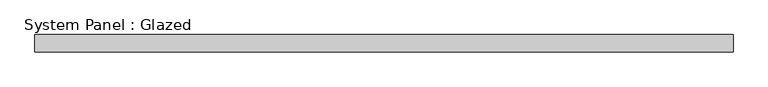
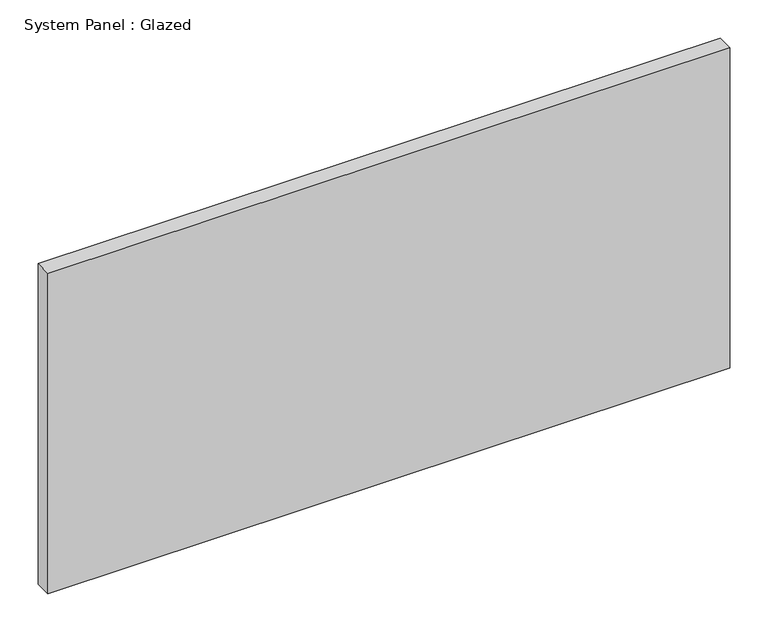
"""IFC4 building model written with IfcOpenShell, lengths in millimetres: plate geometry, System Panel : Glazed."""

from ifc_helpers import new_model, si_unit, origin, origin_with_axes, place, context, project, spatial, polyline, outline, extrude, source, transform, mapped, element, save


def system_panel_glazed_368d4c1c(model_context):
    return source(origin(), model_context, "Body", "SweptSolid", [
        extrude(outline(polyline([(517.525, 19.05), (-517.525, 19.05), (-517.525, 44.45), (517.525, 44.45), (517.525, 19.05)])), origin_with_axes(), (0.0, 0.0, 1.0), 514.35),
    ])


if __name__ == "__main__":
    model = new_model("IFC4")
    model_context = context("Model", 3, world=origin())
    ifc_project = project(units=[si_unit("LENGTHUNIT", "METRE", prefix="MILLI")], contexts=[model_context])
    site = spatial("IfcSite", under=ifc_project)
    building = spatial("IfcBuilding", under=site)
    placement = place(None, origin())
    system_panel_glazed_shape = system_panel_glazed_368d4c1c(model_context)
    element("IfcPlate", 1, ObjectType="System Panel : Glazed", at=placement, inside=building, context=model_context, shape_type="MappedRepresentation", body=[
        mapped(system_panel_glazed_shape, transform((0.0, 0.0, 0.0), x_axis=(1.0, 0.0, 0.0), y_axis=(0.0, 1.0, 0.0), z_axis=(0.0, 0.0, 1.0))),
    ])
    save(model, "model.ifc")

# Revit data of these elements
# Type "System Panel : Glazed"
#   Construction Type Id = "GSP4R"
#   Analytic Construction = "1/8 in Pilkington single glazing"
#   Visual Light Transmittance = 0.9
#   Solar Heat Gain Coefficient = 0.86
#   Heat Transfer Coefficient (U) = 1.18115 BTU/(h·ft²·°F)
#   Define Thermal Properties by = 1
# Element 1 (IfcPlate, "System Panel : Glazed")
#   Materials on its faces: "Glass"
# Materials
#   "Glass": class "Glass", colour RGB 0 128 192, transparency 0.75, Description = "Soda Lime Glass", Cost = 0
